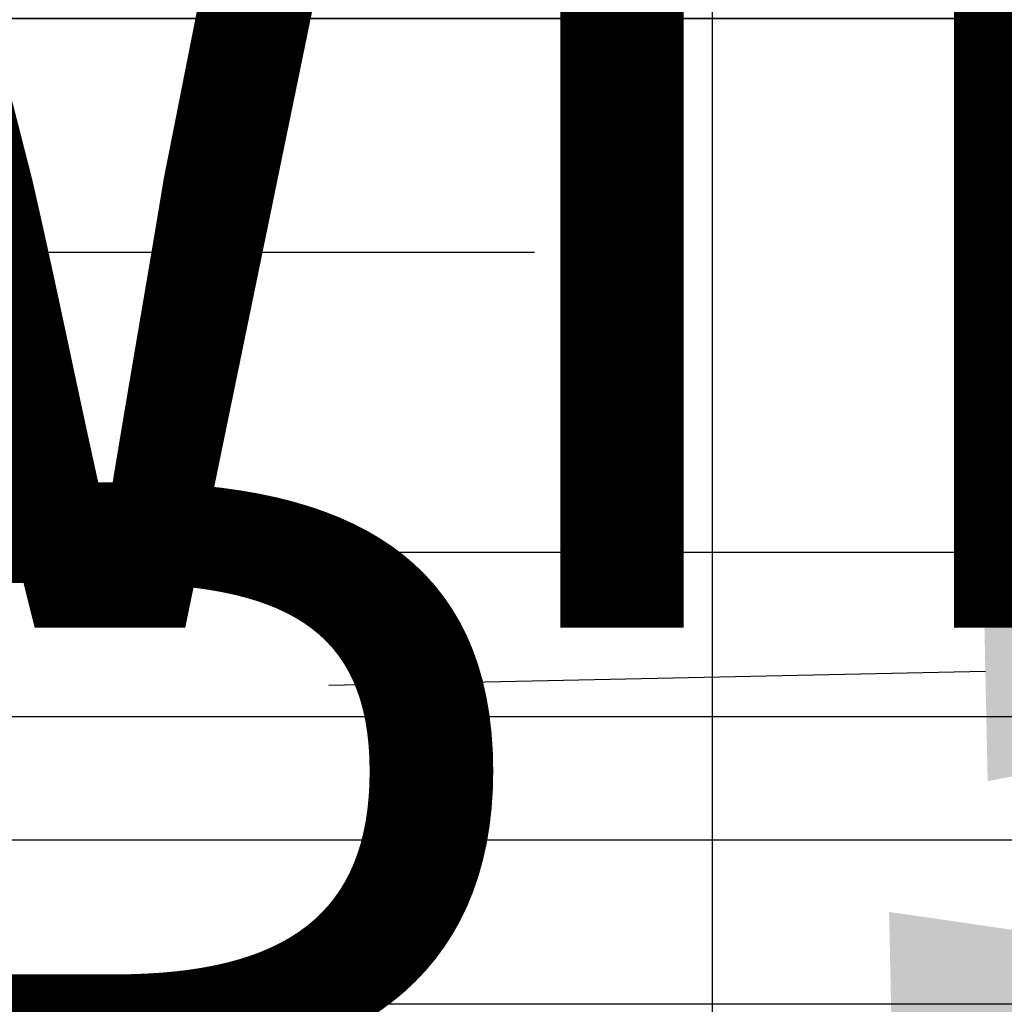
# Model space of a CAD drawing. Units: inches. Extents: x -307 to 2141, y -58 to 895.
# Tile 19 of 28: x 704 to 776, y 517 to 589. Entities that reach past the tile are written whole.
import ezdxf

# ---------------------------------------------------------------- set-up
doc = ezdxf.new("R2010")
doc.units = ezdxf.units.IN
doc.header["$MEASUREMENT"] = 0
doc.layers.add('A-ANNO-DIMS', color=2, linetype='Continuous', lineweight=18)
doc.styles.get("Standard").update_dxf_attribs({"font": 'arial.ttf'})
doc.dimstyles.get("Standard").update_dxf_attribs({"dimtxt": 72, "dimasz": 48, "dimexe": 0.18, "dimexo": 0.0625, "dimgap": 0.09, "dimtad": 0, "dimtih": 1, "dimtoh": 1, "dimdec": 0, "dimrnd": 48, "dimzin": 0, "dimdsep": 46, "dimlunit": 3, "dimtxsty": 'Standard', "dimcen": 0.09, "dimadec": 0, "dimazin": 0, "dimtfac": 1, "dimtdec": 0, "dimtofl": 0, "dimtmove": 0, "dimatfit": 3, "dimfxl": 1, "dimtolj": 1, "dimtzin": 0, "dimarcsym": 0})

# ---------------------------------------------------------------- blocks, each defined once
blk = doc.blocks.new('*D26')
at = {"layer": 'A-ANNO-DIMS', "color": 0, "lineweight": -2, "transparency": 16777216}
for p, q in [((565.336, 584.202), (565.336, 572.085)), ((645.336, 584.202), (645.336, 572.085)), ((517.336, 572.265), (469.336, 572.265)), ((693.336, 572.265), (741.336, 572.265))]:
    blk.add_line(p, q, dxfattribs=at)
at = {"layer": 'A-ANNO-DIMS', "color": 0, "transparency": 16777216}
for points in [[(517.336, 580.265), (517.336, 564.265), (565.336, 572.265)], [(693.336, 580.265), (693.336, 564.265), (645.336, 572.265)]]:
    blk.add_solid(points, dxfattribs=at)
at = {"layer": 'Defpoints', "color": 0, "transparency": 16777216}
for p in [(565.336, 584.265), (645.336, 584.265), (565.336, 572.265)]:
    blk.add_point(p, dxfattribs=at)
at = {"layer": 'A-ANNO-DIMS', "color": 0, "transparency": 16777216, "insert": (178.225, 572.265), "char_height": 72, "attachment_point": 5}
blk.add_mtext('\\A1;BED 80 TYP.', dxfattribs=at)
blk = doc.blocks.new('*D30')
at = {"layer": 'A-ANNO-DIMS', "color": 0, "lineweight": -2, "transparency": 16777216}
for p, q in [((570.736, 532.833), (570.736, 580.833)), ((570.736, 580.833), (618.736, 580.833)), ((565.398, 484.833), (570.916, 484.833)), ((565.398, 448.833), (570.916, 448.833)), ((570.736, 400.833), (570.736, 352.833))]:
    blk.add_line(p, q, dxfattribs=at)
at = {"layer": 'A-ANNO-DIMS', "color": 0, "transparency": 16777216}
for points in [[(562.736, 532.833), (578.736, 532.833), (570.736, 484.833)], [(562.736, 400.833), (578.736, 400.833), (570.736, 448.833)]]:
    blk.add_solid(points, dxfattribs=at)
at = {"layer": 'Defpoints', "color": 0, "transparency": 16777216}
for p in [(565.336, 484.833), (570.736, 484.833), (565.336, 448.833)]:
    blk.add_point(p, dxfattribs=at)
at = {"layer": 'A-ANNO-DIMS', "color": 0, "transparency": 16777216, "insert": (1030.174, 580.833), "char_height": 72, "attachment_point": 5}
blk.add_mtext('\\A1;WINDOW 36 TYP.', dxfattribs=at)
blk = doc.blocks.new('*D31')
at = {"layer": 'A-ANNO-DIMS', "color": 0, "lineweight": -2, "transparency": 16777216}
for p, q in [((556.336, 448.771), (556.336, 443.253)), ((565.336, 448.771), (565.336, 443.253)), ((508.336, 443.433), (460.336, 443.433)), ((613.336, 443.433), (661.336, 443.433))]:
    blk.add_line(p, q, dxfattribs=at)
at = {"layer": 'A-ANNO-DIMS', "color": 0, "transparency": 16777216}
for points in [[(508.336, 451.433), (508.336, 435.433), (556.336, 443.433)], [(613.336, 451.433), (613.336, 435.433), (565.336, 443.433)]]:
    blk.add_solid(points, dxfattribs=at)
at = {"layer": 'Defpoints', "color": 0, "transparency": 16777216}
for p in [(556.336, 448.833), (565.336, 448.833), (565.336, 443.433)]:
    blk.add_point(p, dxfattribs=at)
at = {"layer": 'A-ANNO-DIMS', "color": 0, "transparency": 16777216, "insert": (808.692, 443.433), "char_height": 72, "attachment_point": 5}
blk.add_mtext('\\A1;9 TYP.', dxfattribs=at)
blk = doc.blocks.new('*D32')
at = {"layer": 'A-ANNO-DIMS', "color": 0, "lineweight": -2, "transparency": 16777216}
for p, q in [((813.293, 682.278), (813.293, 671.361)), ((885.293, 682.278), (885.293, 671.361)), ((765.293, 671.541), (717.293, 671.541)), ((933.293, 671.541), (981.293, 671.541))]:
    blk.add_line(p, q, dxfattribs=at)
at = {"layer": 'A-ANNO-DIMS', "color": 0, "transparency": 16777216}
for points in [[(765.293, 679.541), (765.293, 663.541), (813.293, 671.541)], [(933.293, 679.541), (933.293, 663.541), (885.293, 671.541)]]:
    blk.add_solid(points, dxfattribs=at)
at = {"layer": 'Defpoints', "color": 0, "transparency": 16777216}
for p in [(813.293, 682.341), (885.293, 682.341), (885.293, 671.541)]:
    blk.add_point(p, dxfattribs=at)
at = {"layer": 'A-ANNO-DIMS', "color": 0, "transparency": 16777216, "insert": (1392.731, 671.541), "char_height": 72, "attachment_point": 5}
blk.add_mtext('\\A1;WINDOW 72 TYP.', dxfattribs=at)
blk = doc.blocks.new('*D35')
at = {"layer": 'A-ANNO-DIMS', "color": 0, "lineweight": -2, "transparency": 16777216}
for p, q in [((859.336, 453.769), (811.336, 453.769)), ((907.336, 443.029), (907.336, 453.949)), ((916.336, 443.029), (916.336, 453.949)), ((964.336, 453.769), (1012.336, 453.769))]:
    blk.add_line(p, q, dxfattribs=at)
at = {"layer": 'A-ANNO-DIMS', "color": 0, "transparency": 16777216}
for points in [[(859.336, 461.769), (859.336, 445.769), (907.336, 453.769)], [(964.336, 461.769), (964.336, 445.769), (916.336, 453.769)]]:
    blk.add_solid(points, dxfattribs=at)
at = {"layer": 'Defpoints', "color": 0, "transparency": 16777216}
for p in [(907.336, 453.769), (907.336, 442.967), (916.336, 442.967)]:
    blk.add_point(p, dxfattribs=at)
at = {"layer": 'A-ANNO-DIMS', "color": 0, "transparency": 16777216, "insert": (663.98, 453.769), "char_height": 72, "attachment_point": 5}
blk.add_mtext('\\A1;9 TYP.', dxfattribs=at)
blk = doc.blocks.new('*D36')
at = {"layer": 'A-ANNO-DIMS', "color": 0, "lineweight": -2, "transparency": 16777216}
for p, q in [((871.707, 562.404), (871.761, 610.404)), ((876.548, 514.399), (871.474, 514.405)), ((876.511, 481.353), (871.437, 481.358)), ((871.563, 433.358), (871.509, 385.358)), ((871.509, 385.358), (823.509, 385.358))]:
    blk.add_line(p, q, dxfattribs=at)
at = {"layer": 'A-ANNO-DIMS', "color": 0, "transparency": 16777216}
for points in [[(863.707, 562.413), (879.707, 562.395), (871.654, 514.404)], [(863.563, 433.367), (879.563, 433.349), (871.617, 481.358)]]:
    blk.add_solid(points, dxfattribs=at)
at = {"layer": 'Defpoints', "color": 0, "transparency": 16777216}
for p in [(876.611, 514.399), (871.617, 481.358), (876.574, 481.353)]:
    blk.add_point(p, dxfattribs=at)
at = {"layer": 'A-ANNO-DIMS', "color": 0, "transparency": 16777216, "insert": (548.95, 385.358), "char_height": 72, "attachment_point": 5}
blk.add_mtext('\\A1;WC 33 TYP.', dxfattribs=at)
blk = doc.blocks.new('*D37')
at = {"layer": 'A-ANNO-DIMS', "color": 0, "lineweight": -2, "transparency": 16777216}
for p, q in [((828.616, 519.409), (780.616, 519.463)), ((876.611, 514.461), (876.616, 519.536)), ((897.611, 514.438), (897.616, 519.512)), ((945.616, 519.279), (993.616, 519.225))]:
    blk.add_line(p, q, dxfattribs=at)
at = {"layer": 'A-ANNO-DIMS', "color": 0, "transparency": 16777216}
for points in [[(828.625, 527.409), (828.607, 511.409), (876.616, 519.356)], [(945.625, 527.279), (945.607, 511.279), (897.616, 519.332)]]:
    blk.add_solid(points, dxfattribs=at)
at = {"layer": 'Defpoints', "color": 0, "transparency": 16777216}
for p in [(876.616, 519.356), (876.611, 514.399), (897.611, 514.375)]:
    blk.add_point(p, dxfattribs=at)
at = {"layer": 'A-ANNO-DIMS', "color": 0, "transparency": 16777216, "insert": (604.676, 519.463), "char_height": 72, "attachment_point": 5}
blk.add_mtext('\\A1;21 TYP.', dxfattribs=at)
blk = doc.blocks.new('*D42')
at = {"layer": 'A-ANNO-DIMS', "color": 0, "lineweight": -2, "transparency": 16777216}
for p, q in [((880.259, 543.859), (928.248, 544.868)), ((822.302, 541.203), (822.268, 542.82)), ((832.299, 541.413), (832.265, 543.03)), ((774.282, 541.631), (726.293, 540.622))]:
    blk.add_line(p, q, dxfattribs=at)
at = {"layer": 'A-ANNO-DIMS', "color": 0, "transparency": 16777216}
for points in [[(880.09, 551.857), (880.427, 535.861), (832.269, 542.85)], [(774.114, 549.629), (774.45, 533.633), (822.271, 542.64)]]:
    blk.add_solid(points, dxfattribs=at)
at = {"layer": 'Defpoints', "color": 0, "transparency": 16777216}
for p in [(832.269, 542.85), (832.301, 541.35), (822.303, 541.14)]:
    blk.add_point(p, dxfattribs=at)
at = {"layer": 'A-ANNO-DIMS', "color": 0, "transparency": 16777216, "insert": (1192.886, 544.868), "char_height": 72, "attachment_point": 5}
blk.add_mtext('\\A1;FAUCET 10', dxfattribs=at)
blk = doc.blocks.new('*D43')
at = {"layer": 'A-ANNO-DIMS', "color": 0, "lineweight": -2, "transparency": 16777216}
for p, q in [((818.785, 637.088), (770.785, 637.088)), ((819.794, 589.098), (818.785, 637.088)), ((822.24, 541.139), (820.623, 541.105)), ((822.377, 534.64), (820.76, 534.606)), ((821.949, 486.621), (822.958, 438.631))]:
    blk.add_line(p, q, dxfattribs=at)
at = {"layer": 'A-ANNO-DIMS', "color": 0, "transparency": 16777216}
for points in [[(827.792, 589.266), (811.796, 588.93), (820.803, 541.109)], [(829.947, 486.789), (813.951, 486.453), (820.94, 534.61)]]:
    blk.add_solid(points, dxfattribs=at)
at = {"layer": 'Defpoints', "color": 0, "transparency": 16777216}
for p in [(820.803, 541.109), (822.303, 541.14), (822.44, 534.642)]:
    blk.add_point(p, dxfattribs=at)
at = {"layer": 'A-ANNO-DIMS', "color": 0, "transparency": 16777216, "insert": (747.391, 637.088), "char_height": 72, "attachment_point": 5}
blk.add_mtext('\\A1;7', dxfattribs=at)
blk = doc.blocks.new('*D44')
at = {"layer": 'A-ANNO-DIMS', "color": 0, "lineweight": -2, "transparency": 16777216}
for p, q in [((839.872, 521.223), (839.952, 517.424)), ((815.327, 520.707), (815.406, 516.907)), ((887.938, 518.613), (935.927, 519.622)), ((767.413, 516.078), (719.424, 515.069))]:
    blk.add_line(p, q, dxfattribs=at)
at = {"layer": 'A-ANNO-DIMS', "color": 0, "transparency": 16777216}
for points in [[(887.769, 526.611), (888.106, 510.614), (839.948, 517.604)], [(767.245, 524.076), (767.581, 508.08), (815.403, 517.087)]]:
    blk.add_solid(points, dxfattribs=at)
at = {"layer": 'Defpoints', "color": 0, "transparency": 16777216}
for p in [(839.871, 521.285), (815.325, 520.769), (839.948, 517.604)]:
    blk.add_point(p, dxfattribs=at)
at = {"layer": 'A-ANNO-DIMS', "color": 0, "transparency": 16777216, "insert": (1151.157, 519.622), "char_height": 72, "attachment_point": 5}
blk.add_mtext('\\A1;BASIN 25', dxfattribs=at)
blk = doc.blocks.new('*D45')
at = {"layer": 'A-ANNO-DIMS', "color": 0, "lineweight": -2, "transparency": 16777216}
for p, q in [((841.111, 637.474), (793.111, 637.474)), ((842.12, 589.484), (841.111, 637.474)), ((839.51, 541.419), (843.309, 541.499)), ((839.933, 521.287), (843.732, 521.367)), ((844.562, 473.373), (845.571, 425.384))]:
    blk.add_line(p, q, dxfattribs=at)
at = {"layer": 'A-ANNO-DIMS', "color": 0, "transparency": 16777216}
for points in [[(850.118, 589.652), (834.122, 589.316), (843.129, 541.495)], [(852.56, 473.542), (836.563, 473.205), (843.553, 521.363)]]:
    blk.add_solid(points, dxfattribs=at)
at = {"layer": 'Defpoints', "color": 0, "transparency": 16777216}
for p in [(839.447, 541.417), (843.129, 541.495), (839.871, 521.285)]:
    blk.add_point(p, dxfattribs=at)
at = {"layer": 'A-ANNO-DIMS', "color": 0, "transparency": 16777216, "insert": (740.961, 637.474), "char_height": 72, "attachment_point": 5}
blk.add_mtext('\\A1;20', dxfattribs=at)
blk = doc.blocks.new('*D46')
at = {"layer": 'A-ANNO-DIMS', "color": 0, "lineweight": -2, "transparency": 16777216}
for p, q in [((801.413, 645.783), (801.413, 642.516)), ((822.413, 645.783), (822.413, 642.516)), ((753.413, 642.696), (705.413, 642.696)), ((870.413, 642.696), (918.413, 642.696))]:
    blk.add_line(p, q, dxfattribs=at)
at = {"layer": 'A-ANNO-DIMS', "color": 0, "transparency": 16777216}
for points in [[(753.413, 650.696), (753.413, 634.696), (801.413, 642.696)], [(870.413, 650.696), (870.413, 634.696), (822.413, 642.696)]]:
    blk.add_solid(points, dxfattribs=at)
at = {"layer": 'Defpoints', "color": 0, "transparency": 16777216}
for p in [(801.413, 645.846), (822.413, 645.846), (822.413, 642.696)]:
    blk.add_point(p, dxfattribs=at)
at = {"layer": 'A-ANNO-DIMS', "color": 0, "transparency": 16777216, "insert": (1282.702, 642.696), "char_height": 72, "attachment_point": 5}
blk.add_mtext('\\A1;DESK CHAIR 21', dxfattribs=at)
blk = doc.blocks.new('*D52')
at = {"layer": 'A-ANNO-DIMS', "color": 0, "lineweight": -2, "transparency": 16777216}
for p, q in [((660.208, 554.249), (660.208, 602.249)), ((673.796, 506.249), (660.028, 506.249)), ((673.796, 415.249), (660.028, 415.249)), ((660.208, 367.249), (660.208, 319.249))]:
    blk.add_line(p, q, dxfattribs=at)
at = {"layer": 'A-ANNO-DIMS', "color": 0, "transparency": 16777216}
for points in [[(652.208, 554.249), (668.208, 554.249), (660.208, 506.249)], [(652.208, 367.249), (668.208, 367.249), (660.208, 415.249)]]:
    blk.add_solid(points, dxfattribs=at)
at = {"layer": 'Defpoints', "color": 0, "transparency": 16777216}
for p in [(673.858, 506.249), (660.208, 415.249), (673.858, 415.249)]:
    blk.add_point(p, dxfattribs=at)
at = {"layer": 'A-ANNO-DIMS', "color": 0, "transparency": 16777216, "insert": (660.208, 460.749), "char_height": 72, "attachment_point": 5}
blk.add_mtext('\\A1;DINING SET 91', dxfattribs=at)
blk = doc.blocks.new('*D54')
at = {"layer": 'A-ANNO-DIMS', "color": 0, "lineweight": -2, "transparency": 16777216}
for p, q in [((605.336, 412.349), (605.336, 460.349)), ((605.336, 460.349), (653.336, 460.349)), ((596.398, 364.349), (605.516, 364.349)), ((596.398, 304.349), (605.516, 304.349)), ((605.336, 256.349), (605.336, 208.349))]:
    blk.add_line(p, q, dxfattribs=at)
at = {"layer": 'A-ANNO-DIMS', "color": 0, "transparency": 16777216}
for points in [[(597.336, 412.349), (613.336, 412.349), (605.336, 364.349)], [(597.336, 256.349), (613.336, 256.349), (605.336, 304.349)]]:
    blk.add_solid(points, dxfattribs=at)
at = {"layer": 'Defpoints', "color": 0, "transparency": 16777216}
for p in [(596.336, 364.349), (605.336, 364.349), (596.336, 304.349)]:
    blk.add_point(p, dxfattribs=at)
at = {"layer": 'A-ANNO-DIMS', "color": 0, "transparency": 16777216, "insert": (854.004, 460.349), "char_height": 72, "attachment_point": 5}
blk.add_mtext('\\A1;DESK 60', dxfattribs=at)
blk = doc.blocks.new('*D56')
at = {"layer": 'A-ANNO-DIMS', "color": 0, "lineweight": -2, "transparency": 16777216}
for p, q in [((679.732, 723.211), (679.732, 771.211)), ((679.732, 771.211), (727.732, 771.211)), ((675.744, 675.211), (679.912, 675.211)), ((675.744, 648.211), (679.912, 648.211)), ((679.732, 600.211), (679.732, 552.211))]:
    blk.add_line(p, q, dxfattribs=at)
at = {"layer": 'A-ANNO-DIMS', "color": 0, "transparency": 16777216}
for points in [[(671.732, 723.211), (687.732, 723.211), (679.732, 675.211)], [(671.732, 600.211), (687.732, 600.211), (679.732, 648.211)]]:
    blk.add_solid(points, dxfattribs=at)
at = {"layer": 'Defpoints', "color": 0, "transparency": 16777216}
for p in [(675.682, 675.211), (679.732, 675.211), (675.682, 648.211)]:
    blk.add_point(p, dxfattribs=at)
at = {"layer": 'A-ANNO-DIMS', "color": 0, "transparency": 16777216, "insert": (1006.662, 771.211), "char_height": 72, "attachment_point": 5}
blk.add_mtext('\\A1;ROCKER 27', dxfattribs=at)
blk = doc.blocks.new('*D62')
at = {"layer": 'A-ANNO-DIMS', "color": 0, "lineweight": -2, "transparency": 16777216}
for p, q in [((556.336, 691.403), (556.336, 722.725)), ((604.336, 722.545), (656.854, 722.545)), ((868.336, 722.545), (815.817, 722.545)), ((916.336, 490.966), (916.336, 722.725))]:
    blk.add_line(p, q, dxfattribs=at)
at = {"layer": 'A-ANNO-DIMS', "color": 0, "transparency": 16777216}
for points in [[(604.336, 730.545), (604.336, 714.545), (556.336, 722.545)], [(868.336, 730.545), (868.336, 714.545), (916.336, 722.545)]]:
    blk.add_solid(points, dxfattribs=at)
at = {"layer": 'Defpoints', "color": 0, "transparency": 16777216}
for p in [(916.336, 722.545), (556.336, 691.341), (916.336, 490.903)]:
    blk.add_point(p, dxfattribs=at)
at = {"layer": 'A-ANNO-DIMS', "color": 0, "transparency": 16777216, "insert": (736.336, 722.545), "char_height": 72, "attachment_point": 5}
blk.add_mtext('\\A1;360', dxfattribs=at)
blk = doc.blocks.new('*D63')
at = {"layer": 'A-ANNO-DIMS', "color": 0, "lineweight": -2, "transparency": 16777216}
for p, q in [((916.398, 691.341), (947.72, 691.341)), ((947.54, 643.341), (947.54, 416.192)), ((947.54, 115.341), (947.54, 342.49)), ((704.684, 67.341), (947.72, 67.341))]:
    blk.add_line(p, q, dxfattribs=at)
at = {"layer": 'A-ANNO-DIMS', "color": 0, "transparency": 16777216}
for points in [[(939.54, 643.341), (955.54, 643.341), (947.54, 691.341)], [(939.54, 115.341), (955.54, 115.341), (947.54, 67.341)]]:
    blk.add_solid(points, dxfattribs=at)
at = {"layer": 'Defpoints', "color": 0, "transparency": 16777216}
for p in [(916.336, 691.341), (704.621, 67.341), (947.54, 67.341)]:
    blk.add_point(p, dxfattribs=at)
at = {"layer": 'A-ANNO-DIMS', "color": 0, "transparency": 16777216, "insert": (947.54, 379.341), "char_height": 72, "attachment_point": 5}
blk.add_mtext('\\A1;624', dxfattribs=at)
blk = doc.blocks.new('*D68')
at = {"layer": 'A-ANNO-DIMS', "color": 0, "lineweight": -2, "transparency": 16777216}
for p, q in [((525.132, 586.341), (525.132, 634.341)), ((525.132, 634.341), (573.132, 634.341)), ((565.273, 538.341), (524.952, 538.341)), ((556.273, 484.833), (524.952, 484.833)), ((525.132, 436.833), (525.132, 388.833))]:
    blk.add_line(p, q, dxfattribs=at)
at = {"layer": 'A-ANNO-DIMS', "color": 0, "transparency": 16777216}
for points in [[(517.132, 586.341), (533.132, 586.341), (525.132, 538.341)], [(517.132, 436.833), (533.132, 436.833), (525.132, 484.833)]]:
    blk.add_solid(points, dxfattribs=at)
at = {"layer": 'Defpoints', "color": 0, "transparency": 16777216}
for p in [(525.132, 538.341), (565.336, 538.341), (556.336, 484.833)]:
    blk.add_point(p, dxfattribs=at)
at = {"layer": 'A-ANNO-DIMS', "color": 0, "transparency": 16777216, "insert": (687.754, 634.341), "char_height": 72, "attachment_point": 5}
blk.add_mtext('\\A1;53.51', dxfattribs=at)
blk = doc.blocks.new('*D69')
at = {"layer": 'A-ANNO-DIMS', "color": 0, "lineweight": -2, "transparency": 16777216}
for p, q in [((525.132, 682.341), (525.132, 730.341)), ((525.132, 730.341), (573.132, 730.341)), ((565.273, 682.341), (524.952, 682.341)), ((525.132, 586.341), (525.132, 634.341)), ((565.273, 538.341), (524.952, 538.341))]:
    blk.add_line(p, q, dxfattribs=at)
at = {"layer": 'A-ANNO-DIMS', "color": 0, "transparency": 16777216}
for points in [[(517.132, 634.341), (533.132, 634.341), (525.132, 682.341)], [(517.132, 586.341), (533.132, 586.341), (525.132, 538.341)]]:
    blk.add_solid(points, dxfattribs=at)
at = {"layer": 'Defpoints', "color": 0, "transparency": 16777216}
for p in [(525.132, 682.341), (565.336, 682.341), (565.336, 538.341)]:
    blk.add_point(p, dxfattribs=at)
at = {"layer": 'A-ANNO-DIMS', "color": 0, "transparency": 16777216, "insert": (649.225, 730.341), "char_height": 72, "attachment_point": 5}
blk.add_mtext('\\A1;144', dxfattribs=at)
blk = doc.blocks.new('*D78')
at = {"layer": 'A-ANNO-DIMS', "color": 0, "lineweight": -2, "transparency": 16777216}
for p, q in [((947.53984, 730.340828), (947.53984, 778.340828)), ((778.39834, 682.340828), (947.71984, 682.340828)), ((730.39834, 598.340828), (947.71984, 598.340828)), ((947.53984, 550.340828), (947.53984, 502.340828))]:
    blk.add_line(p, q, dxfattribs=at)
at = {"layer": 'A-ANNO-DIMS', "color": 0, "transparency": 16777216}
for points in [[(939.53984, 730.340828), (955.53984, 730.340828), (947.53984, 682.340828)], [(939.53984, 550.340828), (955.53984, 550.340828), (947.53984, 598.340828)]]:
    blk.add_solid(points, dxfattribs=at)
at = {"layer": 'Defpoints', "color": 0, "transparency": 16777216}
for p in [(778.33584, 682.340828), (947.53984, 682.340828), (730.33584, 598.340828)]:
    blk.add_point(p, dxfattribs=at)
at = {"layer": 'A-ANNO-DIMS', "color": 0, "transparency": 16777216, "insert": (947.53984, 640.340828), "char_height": 72, "attachment_point": 5}
blk.add_mtext('\\A1;84', dxfattribs=at)
blk = doc.blocks.new('*D80')
at = {"layer": 'A-ANNO-DIMS', "color": 0, "lineweight": -2, "transparency": 16777216}
for p, q in [((763.336, 722.545), (715.336, 722.545)), ((811.336, 517.403), (811.336, 722.725)), ((907.336, 541.403), (907.336, 722.725)), ((955.336, 722.545), (1003.336, 722.545))]:
    blk.add_line(p, q, dxfattribs=at)
at = {"layer": 'A-ANNO-DIMS', "color": 0, "transparency": 16777216}
for points in [[(763.336, 730.545), (763.336, 714.545), (811.336, 722.545)], [(955.336, 730.545), (955.336, 714.545), (907.336, 722.545)]]:
    blk.add_solid(points, dxfattribs=at)
at = {"layer": 'Defpoints', "color": 0, "transparency": 16777216}
for p in [(907.336, 722.545), (907.336, 541.341), (811.336, 517.341)]:
    blk.add_point(p, dxfattribs=at)
at = {"layer": 'A-ANNO-DIMS', "color": 0, "transparency": 16777216, "insert": (1054.97, 722.545), "char_height": 72, "attachment_point": 5}
blk.add_mtext('\\A1;96', dxfattribs=at)
blk = doc.blocks.new('*D82')
at = {"layer": 'A-ANNO-DIMS', "color": 0, "lineweight": -2, "transparency": 16777216}
for p, q in [((525.132, 565.341), (525.132, 613.341)), ((525.132, 613.341), (573.132, 613.341)), ((802.273, 517.341), (524.952, 517.341)), ((802.273, 481.341), (524.952, 481.341)), ((525.132, 433.341), (525.132, 385.341))]:
    blk.add_line(p, q, dxfattribs=at)
at = {"layer": 'A-ANNO-DIMS', "color": 0, "transparency": 16777216}
for points in [[(517.132, 565.341), (533.132, 565.341), (525.132, 517.341)], [(517.132, 433.341), (533.132, 433.341), (525.132, 481.341)]]:
    blk.add_solid(points, dxfattribs=at)
at = {"layer": 'Defpoints', "color": 0, "transparency": 16777216}
for p in [(525.132, 517.341), (802.336, 517.341), (802.336, 481.341)]:
    blk.add_point(p, dxfattribs=at)
at = {"layer": 'A-ANNO-DIMS', "color": 0, "transparency": 16777216, "insert": (624.742, 613.341), "char_height": 72, "attachment_point": 5}
blk.add_mtext('\\A1;36', dxfattribs=at)
blk = doc.blocks.new('*D83')
at = {"layer": 'A-ANNO-DIMS', "color": 0, "lineweight": -2, "transparency": 16777216}
for p, q in [((947.54, 538.903), (947.54, 586.903)), ((916.398, 490.903), (947.72, 490.903)), ((907.398, 481.341), (947.72, 481.341)), ((947.54, 433.341), (947.54, 385.341)), ((947.54, 385.341), (899.54, 385.341))]:
    blk.add_line(p, q, dxfattribs=at)
at = {"layer": 'A-ANNO-DIMS', "color": 0, "transparency": 16777216}
for points in [[(939.54, 538.903), (955.54, 538.903), (947.54, 490.903)], [(939.54, 433.341), (955.54, 433.341), (947.54, 481.341)]]:
    blk.add_solid(points, dxfattribs=at)
at = {"layer": 'Defpoints', "color": 0, "transparency": 16777216}
for p in [(916.336, 490.903), (907.336, 481.341), (947.54, 481.341)]:
    blk.add_point(p, dxfattribs=at)
at = {"layer": 'A-ANNO-DIMS', "color": 0, "transparency": 16777216, "insert": (777.968, 385.341), "char_height": 72, "attachment_point": 5}
blk.add_mtext('\\A1;9.563', dxfattribs=at)
blk = doc.blocks.new('*D88')
at = {"layer": 'A-ANNO-DIMS', "color": 0, "lineweight": -2, "transparency": 16777216}
for p, q in [((517.33584, 722.544828), (469.33584, 722.544828)), ((565.33584, 295.403328), (565.33584, 722.724828)), ((754.33584, 271.403328), (754.33584, 722.724828)), ((802.33584, 722.544828), (850.33584, 722.544828))]:
    blk.add_line(p, q, dxfattribs=at)
at = {"layer": 'A-ANNO-DIMS', "color": 0, "transparency": 16777216}
for points in [[(517.33584, 730.544828), (517.33584, 714.544828), (565.33584, 722.544828)], [(802.33584, 730.544828), (802.33584, 714.544828), (754.33584, 722.544828)]]:
    blk.add_solid(points, dxfattribs=at)
at = {"layer": 'Defpoints', "color": 0, "transparency": 16777216}
for p in [(754.33584, 722.544828), (565.33584, 295.340828), (754.33584, 271.340828)]:
    blk.add_point(p, dxfattribs=at)
at = {"layer": 'A-ANNO-DIMS', "color": 0, "transparency": 16777216, "insert": (659.83584, 722.544828), "char_height": 72, "attachment_point": 5}
blk.add_mtext('\\A1;189', dxfattribs=at)
blk = doc.blocks.new('*D94')
at = {"layer": 'A-ANNO-DIMS', "color": 0, "lineweight": -2, "transparency": 16777216}
for p, q in [((517.336, 722.545), (469.336, 722.545)), ((565.336, 529.403), (565.336, 722.725)), ((629.836, 529.403), (629.836, 722.725)), ((677.836, 722.545), (725.836, 722.545))]:
    blk.add_line(p, q, dxfattribs=at)
at = {"layer": 'A-ANNO-DIMS', "color": 0, "transparency": 16777216}
for points in [[(517.336, 730.545), (517.336, 714.545), (565.336, 722.545)], [(677.836, 730.545), (677.836, 714.545), (629.836, 722.545)]]:
    blk.add_solid(points, dxfattribs=at)
at = {"layer": 'Defpoints', "color": 0, "transparency": 16777216}
for p in [(629.836, 722.545), (565.336, 529.341), (629.836, 529.341)]:
    blk.add_point(p, dxfattribs=at)
at = {"layer": 'A-ANNO-DIMS', "color": 0, "transparency": 16777216, "insert": (819.904, 722.545), "char_height": 72, "attachment_point": 5}
blk.add_mtext('\\A1;64.5', dxfattribs=at)
blk = doc.blocks.new('*D95')
at = {"layer": 'A-ANNO-DIMS', "color": 0, "lineweight": -2, "transparency": 16777216}
for p, q in [((947.54, 577.341), (947.54, 625.341)), ((947.54, 625.341), (995.54, 625.341)), ((629.898, 529.341), (947.72, 529.341)), ((629.898, 502.663), (947.72, 502.663)), ((947.54, 454.663), (947.54, 406.663))]:
    blk.add_line(p, q, dxfattribs=at)
at = {"layer": 'A-ANNO-DIMS', "color": 0, "transparency": 16777216}
for points in [[(939.54, 577.341), (955.54, 577.341), (947.54, 529.341)], [(939.54, 454.663), (955.54, 454.663), (947.54, 502.663)]]:
    blk.add_solid(points, dxfattribs=at)
at = {"layer": 'Defpoints', "color": 0, "transparency": 16777216}
for p in [(629.836, 529.341), (947.54, 529.341), (629.836, 502.663)]:
    blk.add_point(p, dxfattribs=at)
at = {"layer": 'A-ANNO-DIMS', "color": 0, "transparency": 16777216, "insert": (1117.799, 625.341), "char_height": 72, "attachment_point": 5}
blk.add_mtext('\\A1;26.68', dxfattribs=at)
blk = doc.blocks.new('*D97')
at = {"layer": 'A-ANNO-DIMS', "color": 0, "lineweight": -2, "transparency": 16777216}
for p, q in [((947.54, 637.341), (947.54, 685.341)), ((947.54, 685.341), (995.54, 685.341)), ((685.398, 589.341), (947.72, 589.341)), ((685.398, 538.341), (947.72, 538.341)), ((947.54, 490.341), (947.54, 442.341))]:
    blk.add_line(p, q, dxfattribs=at)
at = {"layer": 'A-ANNO-DIMS', "color": 0, "transparency": 16777216}
for points in [[(939.54, 637.341), (955.54, 637.341), (947.54, 589.341)], [(939.54, 490.341), (955.54, 490.341), (947.54, 538.341)]]:
    blk.add_solid(points, dxfattribs=at)
at = {"layer": 'Defpoints', "color": 0, "transparency": 16777216}
for p in [(685.336, 589.341), (947.54, 589.341), (685.336, 538.341)]:
    blk.add_point(p, dxfattribs=at)
at = {"layer": 'A-ANNO-DIMS', "color": 0, "transparency": 16777216, "insert": (1040.249, 685.341), "char_height": 72, "attachment_point": 5}
blk.add_mtext('\\A1;51', dxfattribs=at)
blk = doc.blocks.new('*D98')
at = {"layer": 'A-ANNO-DIMS', "color": 0, "lineweight": -2, "transparency": 16777216}
for p, q in [((525.132, 637.341), (525.132, 685.341)), ((525.132, 685.341), (573.132, 685.341)), ((787.273, 589.341), (524.952, 589.341)), ((787.273, 550.341), (524.952, 550.341)), ((525.132, 502.341), (525.132, 454.341))]:
    blk.add_line(p, q, dxfattribs=at)
at = {"layer": 'A-ANNO-DIMS', "color": 0, "transparency": 16777216}
for points in [[(517.132, 637.341), (533.132, 637.341), (525.132, 589.341)], [(517.132, 502.341), (533.132, 502.341), (525.132, 550.341)]]:
    blk.add_solid(points, dxfattribs=at)
at = {"layer": 'Defpoints', "color": 0, "transparency": 16777216}
for p in [(525.132, 589.341), (787.336, 589.341), (787.336, 550.341)]:
    blk.add_point(p, dxfattribs=at)
at = {"layer": 'A-ANNO-DIMS', "color": 0, "transparency": 16777216, "insert": (624.84, 685.341), "char_height": 72, "attachment_point": 5}
blk.add_mtext('\\A1;39', dxfattribs=at)
blk = doc.blocks.new('*D107')
at = {"layer": 'A-ANNO-DIMS', "color": 0, "lineweight": -2, "transparency": 16777216}
for p, q in [((517.336, 722.545), (469.336, 722.545)), ((565.336, 409.403), (565.336, 722.725)), ((589.339, 409.403), (589.339, 722.725)), ((637.339, 722.545), (685.339, 722.545))]:
    blk.add_line(p, q, dxfattribs=at)
at = {"layer": 'A-ANNO-DIMS', "color": 0, "transparency": 16777216}
for points in [[(517.336, 730.545), (517.336, 714.545), (565.336, 722.545)], [(637.339, 730.545), (637.339, 714.545), (589.339, 722.545)]]:
    blk.add_solid(points, dxfattribs=at)
at = {"layer": 'Defpoints', "color": 0, "transparency": 16777216}
for p in [(589.339, 722.545), (565.336, 409.341), (589.339, 409.341)]:
    blk.add_point(p, dxfattribs=at)
at = {"layer": 'A-ANNO-DIMS', "color": 0, "transparency": 16777216, "insert": (835.495, 722.545), "char_height": 72, "attachment_point": 5}
blk.add_mtext('\\A1;24.003', dxfattribs=at)
blk = doc.blocks.new('*D108')
at = {"layer": 'A-ANNO-DIMS', "color": 0, "lineweight": -2, "transparency": 16777216}
for p, q in [((947.54, 550.663), (947.54, 598.663)), ((589.402, 502.663), (947.72, 502.663)), ((589.402, 409.341), (947.72, 409.341)), ((947.54, 361.341), (947.54, 313.341))]:
    blk.add_line(p, q, dxfattribs=at)
at = {"layer": 'A-ANNO-DIMS', "color": 0, "transparency": 16777216}
for points in [[(939.54, 550.663), (955.54, 550.663), (947.54, 502.663)], [(939.54, 361.341), (955.54, 361.341), (947.54, 409.341)]]:
    blk.add_solid(points, dxfattribs=at)
at = {"layer": 'Defpoints', "color": 0, "transparency": 16777216}
for p in [(589.339, 502.663), (947.54, 502.663), (589.339, 409.341)]:
    blk.add_point(p, dxfattribs=at)
at = {"layer": 'A-ANNO-DIMS', "color": 0, "transparency": 16777216, "insert": (947.54, 456.002), "char_height": 72, "attachment_point": 5}
blk.add_mtext('\\A1;93.32', dxfattribs=at)

msp = doc.modelspace()

# ---------------------------------------------------------------- dimensions: what is measured, and where the dimension line sits
at = {"layer": 'A-ANNO-DIMS'}
for base, p1, p2, angle, text, picture, middle in [((679.7317, 675.211), (675.6817, 648.211), (675.6817, 675.211), 90, 'ROCKER <>', '*D56', (1006.6621, 771.211)), ((570.7358, 484.8333), (565.3358, 448.8333), (565.3358, 484.8333), 90, 'WINDOW <> TYP.', '*D30', (1030.1737, 580.8333)), ((565.3358, 572.2648), (645.3359, 584.2648), (565.3358, 584.2648), 180, 'BED <> TYP.', '*D26', (178.2254, 572.2648)), ((832.2692, 542.8502), (822.3029, 541.1403), (832.3007, 541.3505), 1.204628, 'FAUCET <>', '*D42', (1192.8864, 544.8684)), ((660.2083, 415.2485), (673.8583, 506.2485), (673.8583, 415.2485), 270, 'DINING SET <>', '*D52', (660.2083, 460.7485)), ((876.6162, 519.3557), (897.6106, 514.3753), (876.6106, 514.3988), 179.935892, '<> TYP.', '*D37', (604.6763, 519.4631)), ((839.9481, 517.6035), (815.3253, 520.7692), (839.8707, 521.2853), 1.204628, 'BASIN <>', '*D44', (1151.1574, 519.6217)), ((871.6167, 481.3581), (876.6106, 514.3988), (876.5736, 481.3526), 269.935892, 'WC <> TYP.', '*D36', (548.95, 385.3582)), ((605.3358, 364.3488), (596.3358, 304.3488), (596.3358, 364.3488), 90, 'DESK <>', '*D54', (854.0043, 460.3488)), ((907.3358, 453.7692), (916.3358, 442.9669), (907.3358, 442.9669), 180, '<> TYP.', '*D35', (663.9798, 453.7692))]:
    dim = msp.add_linear_dim(base=base, p1=p1, p2=p2, angle=angle, text=text, dimstyle='Standard', override={"dimdec": 0, "dimlfac": 1, "dimrnd": 0, "dimzin": 0, "dimdsep": 46, "dimlunit": 2}, dxfattribs=at)
    dim.commit()
    dim.dimension.update_dxf_attribs({"geometry": picture, "text_midpoint": middle})
for base, p1, p2, text, picture, middle in [((885.2934, 671.5408), (813.2934, 682.3408), (885.2934, 682.3408), 'WINDOW <> TYP.', '*D32', (1392.7312, 671.5408)), ((822.4132, 642.696), (801.4132, 645.846), (822.4132, 645.846), 'DESK CHAIR <>', '*D46', (1282.7024, 642.696)), ((565.3358, 443.4333), (556.3358, 448.8333), (565.3358, 448.8333), '<> TYP.', '*D31', (808.6919, 443.4333))]:
    dim = msp.add_linear_dim(base=base, p1=p1, p2=p2, text=text, dimstyle='Standard', override={"dimdec": 0, "dimlfac": 1, "dimrnd": 0, "dimzin": 0, "dimdsep": 46, "dimlunit": 2}, dxfattribs=at)
    dim.commit()
    dim.dimension.update_dxf_attribs({"geometry": picture, "text_midpoint": middle})
for base, p1, p2, angle, override, picture, middle in [((947.5398, 682.3408), (730.3358, 598.3408), (778.3358, 682.3408), 90, {"dimdec": 0, "dimlfac": 1, "dimrnd": 0, "dimzin": 0, "dimdsep": 46, "dimlunit": 2}, '*D78', (947.5398, 640.3408)), ((525.1318, 682.3408), (565.3358, 538.3408), (565.3358, 682.3408), 90, {"dimdec": 0, "dimlfac": 1, "dimrnd": 0, "dimzin": 0, "dimdsep": 46, "dimlunit": 2}, '*D69', (649.2246, 730.3408)), ((525.1318, 589.3408), (787.3358, 550.3408), (787.3358, 589.3408), 90, {"dimdec": 0, "dimlfac": 1, "dimrnd": 0, "dimzin": 0, "dimdsep": 46, "dimlunit": 2}, '*D98', (624.8398, 685.3408)), ((947.5398, 589.3408), (685.3358, 538.3408), (685.3358, 589.3408), 90, {"dimdec": 0, "dimlfac": 1, "dimrnd": 0, "dimzin": 0, "dimdsep": 46, "dimlunit": 2}, '*D97', (1040.2492, 685.3408)), ((947.5398, 67.3408), (916.3358, 691.3408), (704.6211, 67.3408), 90, {"dimdec": 0, "dimlfac": 1, "dimrnd": 0, "dimzin": 0, "dimdsep": 46, "dimlunit": 2}, '*D63', (947.5398, 379.3408)), ((843.1292, 541.4949), (839.8707, 521.2853), (839.4474, 541.4175), 91.204628, {"dimdec": 0, "dimlfac": 1, "dimrnd": 0, "dimzin": 0, "dimdsep": 46, "dimlunit": 2}, '*D45', (740.961, 637.4737)), ((820.8033, 541.1087), (822.4396, 534.6416), (822.3029, 541.1403), 91.204628, {"dimdec": 0, "dimlfac": 1, "dimrnd": 0, "dimzin": 0, "dimdsep": 46, "dimlunit": 2}, '*D43', (747.3908, 637.0875)), ((525.1318, 538.3408), (556.3358, 484.8333), (565.3358, 538.3408), 90, {"dimdec": 2, "dimlfac": 1, "dimrnd": 0, "dimzin": 0, "dimdsep": 46, "dimlunit": 2}, '*D68', (687.7539, 634.3408)), ((947.5398, 529.3408), (629.8358, 502.6632), (629.8358, 529.3408), 90, {"dimdec": 2, "dimlfac": 1, "dimrnd": 0, "dimzin": 0, "dimdsep": 46, "dimlunit": 2}, '*D95', (1117.799, 625.3408)), ((525.1318, 517.3408), (802.3358, 481.3408), (802.3358, 517.3408), 90, {"dimdec": 0, "dimlfac": 1, "dimrnd": 0, "dimzin": 0, "dimdsep": 46, "dimlunit": 2}, '*D82', (624.7416, 613.3408)), ((947.5398, 502.6632), (589.339, 409.3408), (589.339, 502.6632), 90, {"dimdec": 2, "dimlfac": 1, "dimrnd": 0, "dimzin": 0, "dimdsep": 46, "dimlunit": 2}, '*D108', (947.5398, 456.002)), ((947.5398, 481.3408), (916.3358, 490.9034), (907.3358, 481.3408), 90, {"dimdec": 3, "dimlfac": 1, "dimrnd": 0, "dimzin": 0, "dimdsep": 46, "dimlunit": 2}, '*D83', (777.9683, 385.3408))]:
    dim = msp.add_linear_dim(base=base, p1=p1, p2=p2, angle=angle, dimstyle='Standard', override=override, dxfattribs=at)
    dim.commit()
    dim.dimension.update_dxf_attribs({"geometry": picture, "text_midpoint": middle})
for base, p1, p2, override, picture, middle in [((754.3358, 722.5448), (565.3358, 295.3408), (754.3358, 271.3408), {"dimdec": 0, "dimlfac": 1, "dimrnd": 0, "dimzin": 0, "dimdsep": 46, "dimlunit": 2}, '*D88', (659.8358, 722.5448)), ((629.8358, 722.5448), (565.3358, 529.3408), (629.8358, 529.3408), {"dimdec": 1, "dimlfac": 1, "dimrnd": 0, "dimzin": 0, "dimdsep": 46, "dimlunit": 2}, '*D94', (819.904, 722.5448)), ((589.339, 722.5448), (565.3358, 409.3408), (589.339, 409.3408), {"dimdec": 3, "dimlfac": 1, "dimrnd": 0, "dimzin": 0, "dimdsep": 46, "dimlunit": 2}, '*D107', (835.4945, 722.5448)), ((916.3358, 722.5448), (556.3358, 691.3408), (916.3358, 490.9034), {"dimdec": 0, "dimlfac": 1, "dimrnd": 0, "dimzin": 0, "dimdsep": 46, "dimlunit": 2}, '*D62', (736.3358, 722.5448)), ((907.3358, 722.5448), (811.3358, 517.3408), (907.3358, 541.3408), {"dimdec": 0, "dimlfac": 1, "dimrnd": 0, "dimzin": 0, "dimdsep": 46, "dimlunit": 2}, '*D80', (1054.9702, 722.5448))]:
    dim = msp.add_linear_dim(base=base, p1=p1, p2=p2, dimstyle='Standard', override=override, dxfattribs=at)
    dim.commit()
    dim.dimension.update_dxf_attribs({"geometry": picture, "text_midpoint": middle})

doc.saveas('drawing.dxf')
